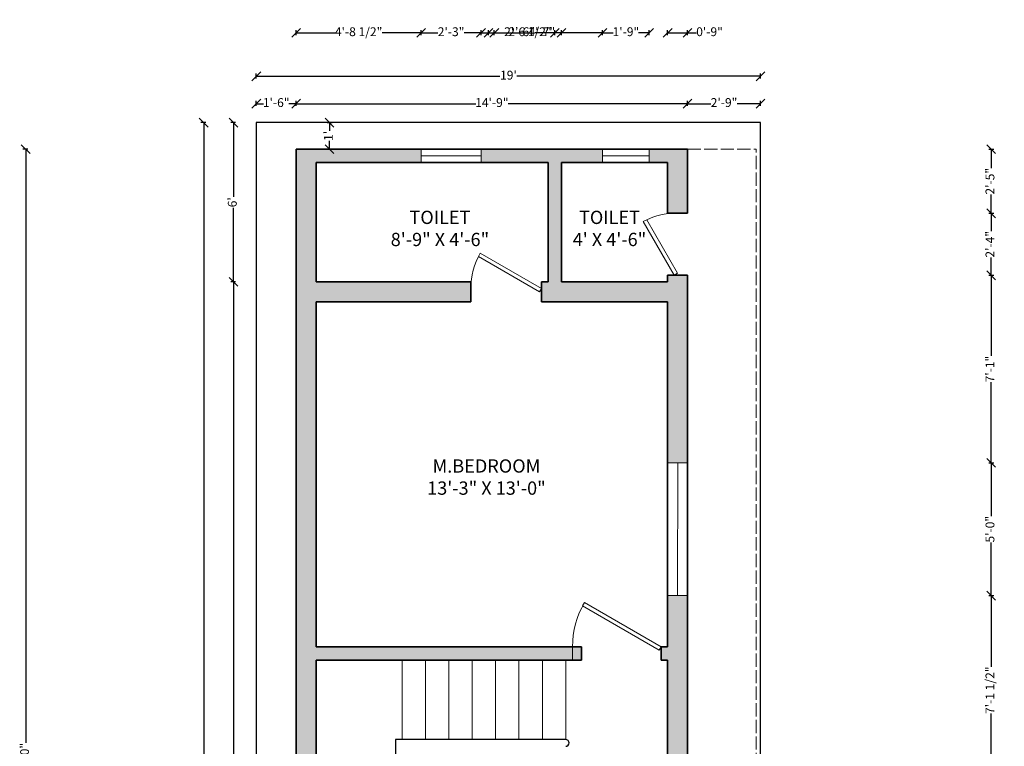
# Model space of a CAD drawing. Units: inches. Extents: x 2349 to 2798, y 397 to 1271.
# Tile 3 of 3: x 2353 to 2798, y 943 to 1271. Entities that reach past the tile are written whole.
import ezdxf

# ---------------------------------------------------------------- set-up
doc = ezdxf.new("R2010")
doc.units = ezdxf.units.IN
doc.linetypes.add('ACAD_ISO02W100', pattern=[15, 12, -3])
for name, color, linetype, lineweight in [('A-ANNO-DIMS', 2, 'Continuous', 18), ('A-AREA-IDEN', 7, 'Continuous', 18), ('A-DOOR', 4, 'Continuous', 18), ('A-FLOR-HRAL', 132, 'Continuous', 25), ('A-FLOR-OVHD', 253, 'ACAD_ISO02W100', 13), ('A-FLOR-STRS', 8, 'Continuous', 18), ('A-GLAZ', 4, 'Continuous', 18), ('A-WALL', 7, 'Continuous', 35), ('A-WALL-PATT', 8, 'Continuous', 13), ('C-PROP', 7, 'Continuous', 25)]:
    doc.layers.add(name, color=color, linetype=linetype, lineweight=lineweight)
doc.styles.get("Standard").update_dxf_attribs({"font": 'arial.ttf'})
doc.dimstyles.new('ISO-25', dxfattribs={"dimtxt": 4, "dimasz": 4, "dimexe": 1.25, "dimexo": 1, "dimtad": 0, "dimdec": 1, "dimlunit": 3, "dimtxsty": 'Standard', "dimblk": 'OBLIQUE', "dimcen": 2.5, "dimclrd": 1, "dimclrt": 3, "dimadec": 0, "dimazin": 0, "dimtfac": 1, "dimtdec": 1, "dimtmove": 0, "dimatfit": 3, "dimfxl": 1, "dimfxlon": 1, "dimarcsym": 0})

# ---------------------------------------------------------------- blocks, each defined once
blk = doc.blocks.new('_Oblique')
at = {"color": 0, "linetype": 'ByBlock', "lineweight": -2}
blk.add_line((-0.5, -0.5), (0.5, 0.5), dxfattribs=at)
blk = doc.blocks.new('*D2')
at = {"layer": 'A-ANNO-DIMS', "color": 0, "lineweight": -2, "transparency": 16777216}
for p, q in [((2491.82, 1224.52), (2494.07, 1224.52)), ((2492.82, 1224.52), (2492.82, 1220.79)), ((2492.82, 1212.52), (2492.82, 1216.24)), ((2491.82, 1212.52), (2494.07, 1212.52))]:
    blk.add_line(p, q, dxfattribs=at)
at = {"layer": 'Defpoints', "color": 0, "transparency": 16777216}
for p in [(2477.73, 1224.52), (2492.82, 1224.52), (2477.73, 1212.52)]:
    blk.add_point(p, dxfattribs=at)
at = {"layer": 'A-ANNO-DIMS', "color": 0, "lineweight": -2, "transparency": 16777216, "xscale": 4, "yscale": 4, "zscale": 4}
for p, rotation in [((2492.82, 1224.52), 90), ((2492.82, 1212.52), 270)]:
    blk.add_blockref('_Oblique', p, dxfattribs=dict(at, rotation=rotation))
at = {"layer": 'A-ANNO-DIMS', "color": 0, "transparency": 16777216, "insert": (2492.82, 1218.52), "char_height": 4, "attachment_point": 5, "rotation": 90}
blk.add_mtext("1'", dxfattribs=at)
blk = doc.blocks.new('*D3')
at = {"layer": 'A-ANNO-DIMS', "color": 0, "lineweight": -2, "transparency": 16777216}
for p, q in [((2459.73, 1232.09), (2459.73, 1234.34)), ((2477.73, 1232.09), (2477.73, 1234.34)), ((2459.73, 1233.09), (2462.98, 1233.09)), ((2477.73, 1233.09), (2474.48, 1233.09))]:
    blk.add_line(p, q, dxfattribs=at)
at = {"layer": 'Defpoints', "color": 0, "transparency": 16777216}
for p in [(2477.73, 1233.09), (2459.73, 1224.52), (2477.73, 1224.52)]:
    blk.add_point(p, dxfattribs=at)
at = {"layer": 'A-ANNO-DIMS', "color": 0, "lineweight": -2, "transparency": 16777216, "xscale": 4, "yscale": 4, "zscale": 4, "rotation": 180}
blk.add_blockref('_Oblique', (2459.73, 1233.09), dxfattribs=at)
at = {"layer": 'A-ANNO-DIMS', "color": 0, "lineweight": -2, "transparency": 16777216, "xscale": 4, "yscale": 4, "zscale": 4}
blk.add_blockref('_Oblique', (2477.73, 1233.09), dxfattribs=at)
at = {"layer": 'A-ANNO-DIMS', "color": 0, "transparency": 16777216, "insert": (2468.73, 1233.09), "char_height": 4, "attachment_point": 5}
blk.add_mtext('1\'-6"', dxfattribs=at)
blk = doc.blocks.new('*D4')
at = {"layer": 'A-ANNO-DIMS', "color": 0, "lineweight": -2, "transparency": 16777216}
for p, q in [((2477.73, 1232.09), (2477.73, 1234.34)), ((2654.73, 1232.09), (2654.73, 1234.34)), ((2477.73, 1233.09), (2558.92, 1233.09)), ((2654.73, 1233.09), (2573.54, 1233.09))]:
    blk.add_line(p, q, dxfattribs=at)
at = {"layer": 'Defpoints', "color": 0, "transparency": 16777216}
for p in [(2654.73, 1233.09), (2477.73, 1224.52), (2654.73, 1226.53)]:
    blk.add_point(p, dxfattribs=at)
at = {"layer": 'A-ANNO-DIMS', "color": 0, "lineweight": -2, "transparency": 16777216, "xscale": 4, "yscale": 4, "zscale": 4, "rotation": 180}
blk.add_blockref('_Oblique', (2477.73, 1233.09), dxfattribs=at)
at = {"layer": 'A-ANNO-DIMS', "color": 0, "lineweight": -2, "transparency": 16777216, "xscale": 4, "yscale": 4, "zscale": 4}
blk.add_blockref('_Oblique', (2654.73, 1233.09), dxfattribs=at)
at = {"layer": 'A-ANNO-DIMS', "color": 0, "transparency": 16777216, "insert": (2566.23, 1233.09), "char_height": 4, "attachment_point": 5}
blk.add_mtext('14\'-9"', dxfattribs=at)
blk = doc.blocks.new('*D5')
at = {"layer": 'A-ANNO-DIMS', "color": 0, "lineweight": -2, "transparency": 16777216}
for p, q in [((2654.73, 1232.09), (2654.73, 1234.34)), ((2687.73, 1232.09), (2687.73, 1234.34)), ((2654.73, 1233.09), (2665.26, 1233.09)), ((2687.73, 1233.09), (2677.21, 1233.09))]:
    blk.add_line(p, q, dxfattribs=at)
at = {"layer": 'Defpoints', "color": 0, "transparency": 16777216}
for p in [(2687.73, 1233.09), (2654.73, 1226.53), (2687.73, 1224.52)]:
    blk.add_point(p, dxfattribs=at)
at = {"layer": 'A-ANNO-DIMS', "color": 0, "lineweight": -2, "transparency": 16777216, "xscale": 4, "yscale": 4, "zscale": 4, "rotation": 180}
blk.add_blockref('_Oblique', (2654.73, 1233.09), dxfattribs=at)
at = {"layer": 'A-ANNO-DIMS', "color": 0, "lineweight": -2, "transparency": 16777216, "xscale": 4, "yscale": 4, "zscale": 4}
blk.add_blockref('_Oblique', (2687.73, 1233.09), dxfattribs=at)
at = {"layer": 'A-ANNO-DIMS', "color": 0, "transparency": 16777216, "insert": (2671.23, 1233.09), "char_height": 4, "attachment_point": 5}
blk.add_mtext('2\'-9"', dxfattribs=at)
blk = doc.blocks.new('*D6')
at = {"layer": 'A-ANNO-DIMS', "color": 0, "lineweight": -2, "transparency": 16777216}
for p, q in [((2459.73, 1244.48), (2459.73, 1246.73)), ((2687.73, 1244.48), (2687.73, 1246.73)), ((2459.73, 1245.48), (2569.9, 1245.48)), ((2687.73, 1245.48), (2577.56, 1245.48))]:
    blk.add_line(p, q, dxfattribs=at)
at = {"layer": 'Defpoints', "color": 0, "transparency": 16777216}
for p in [(2687.73, 1245.48), (2459.73, 1224.52), (2687.73, 1224.52)]:
    blk.add_point(p, dxfattribs=at)
at = {"layer": 'A-ANNO-DIMS', "color": 0, "lineweight": -2, "transparency": 16777216, "xscale": 4, "yscale": 4, "zscale": 4, "rotation": 180}
blk.add_blockref('_Oblique', (2459.73, 1245.48), dxfattribs=at)
at = {"layer": 'A-ANNO-DIMS', "color": 0, "lineweight": -2, "transparency": 16777216, "xscale": 4, "yscale": 4, "zscale": 4}
blk.add_blockref('_Oblique', (2687.73, 1245.48), dxfattribs=at)
at = {"layer": 'A-ANNO-DIMS', "color": 0, "transparency": 16777216, "insert": (2573.73, 1245.48), "char_height": 4, "attachment_point": 5}
blk.add_mtext("19'", dxfattribs=at)
blk = doc.blocks.new('*D7')
at = {"layer": 'A-ANNO-DIMS', "color": 0, "lineweight": -2, "transparency": 16777216}
for p, q in [((2450.39, 1224.52), (2448.14, 1224.52)), ((2449.39, 1224.52), (2449.39, 1190.99)), ((2449.39, 1152.52), (2449.39, 1186.04)), ((2450.39, 1152.52), (2448.14, 1152.52))]:
    blk.add_line(p, q, dxfattribs=at)
at = {"layer": 'Defpoints', "color": 0, "transparency": 16777216}
for p in [(2459.73, 1224.52), (2449.39, 1152.52), (2459.73, 1152.52)]:
    blk.add_point(p, dxfattribs=at)
at = {"layer": 'A-ANNO-DIMS', "color": 0, "lineweight": -2, "transparency": 16777216, "xscale": 4, "yscale": 4, "zscale": 4}
for p, rotation in [((2449.39, 1224.52), 90), ((2449.39, 1152.52), 270)]:
    blk.add_blockref('_Oblique', p, dxfattribs=dict(at, rotation=rotation))
at = {"layer": 'A-ANNO-DIMS', "color": 0, "transparency": 16777216, "insert": (2449.39, 1188.52), "char_height": 4, "attachment_point": 5, "rotation": 90}
blk.add_mtext("6'", dxfattribs=at)
blk = doc.blocks.new('*D8')
at = {"layer": 'A-ANNO-DIMS', "color": 0, "lineweight": -2, "transparency": 16777216}
for p, q in [((2450.39, 1152.52), (2448.14, 1152.52)), ((2449.39, 1152.52), (2449.39, 914.09)), ((2449.39, 660.52), (2449.39, 898.94)), ((2448.39, 660.52), (2450.64, 660.52))]:
    blk.add_line(p, q, dxfattribs=at)
at = {"layer": 'Defpoints', "color": 0, "transparency": 16777216}
for p in [(2459.73, 1152.52), (2435.42, 660.52), (2449.39, 660.52)]:
    blk.add_point(p, dxfattribs=at)
at = {"layer": 'A-ANNO-DIMS', "color": 0, "lineweight": -2, "transparency": 16777216, "xscale": 4, "yscale": 4, "zscale": 4}
for p, rotation in [((2449.39, 1152.52), 90), ((2449.39, 660.52), 270)]:
    blk.add_blockref('_Oblique', p, dxfattribs=dict(at, rotation=rotation))
at = {"layer": 'A-ANNO-DIMS', "color": 0, "transparency": 16777216, "insert": (2449.39, 906.52), "char_height": 4, "attachment_point": 5, "rotation": 90}
blk.add_mtext('40\'-6"', dxfattribs=at)
blk = doc.blocks.new('*D10')
at = {"layer": 'A-ANNO-DIMS', "color": 0, "lineweight": -2, "transparency": 16777216}
for p, q in [((2436.96, 1224.52), (2434.71, 1224.52)), ((2435.96, 1224.52), (2435.96, 868.55)), ((2435.96, 504.52), (2435.96, 860.49)), ((2436.96, 504.52), (2434.71, 504.52))]:
    blk.add_line(p, q, dxfattribs=at)
at = {"layer": 'Defpoints', "color": 0, "transparency": 16777216}
for p in [(2459.73, 1224.52), (2435.96, 504.52), (2459.73, 504.52)]:
    blk.add_point(p, dxfattribs=at)
at = {"layer": 'A-ANNO-DIMS', "color": 0, "lineweight": -2, "transparency": 16777216, "xscale": 4, "yscale": 4, "zscale": 4}
for p, rotation in [((2435.96, 1224.52), 90), ((2435.96, 504.52), 270)]:
    blk.add_blockref('_Oblique', p, dxfattribs=dict(at, rotation=rotation))
at = {"layer": 'A-ANNO-DIMS', "color": 0, "transparency": 16777216, "insert": (2435.96, 864.52), "char_height": 4, "attachment_point": 5, "rotation": 90}
blk.add_mtext("60'", dxfattribs=at)
blk = doc.blocks.new('*U13')
for p, q in [((0, 0), (0, -6)), ((28, 0), (28, -6))]:
    blk.add_line(p, q)
blk.add_lwpolyline([(0, 0), (24.25, 14), (25.12, 12.48), (0.87, -1.52)], close=True)
blk.add_arc((0, 0), 28, 0, 30)
blk = doc.blocks.new('*U14')
for p, q in [((0, 0), (0, -6)), ((-40, 0), (-40, -6))]:
    blk.add_line(p, q)
blk.add_lwpolyline([(0, 0), (-34.64, 20), (-35.52, 18.48), (-0.88, -1.52)], close=True)
blk.add_arc((0, 0), 40, 150, 180)
blk = doc.blocks.new('*U17')
for p, q in [((0, 0), (0, -6)), ((-32, 0), (-32, -6))]:
    blk.add_line(p, q)
blk.add_lwpolyline([(0, 0), (-27.71, 16), (-28.59, 14.48), (-0.88, -1.52)], close=True)
blk.add_arc((0, 0), 32, 150, 180)
blk = doc.blocks.new('*D19')
at = {"layer": 'A-ANNO-DIMS', "color": 0, "lineweight": -2, "transparency": 16777216}
for p, q in [((2356.46, 1212.52), (2354.21, 1212.52)), ((2356.46, 660.52), (2354.21, 660.52))]:
    blk.add_line(p, q, dxfattribs=at)
at = {"layer": 'A-ANNO-DIMS', "color": 1, "lineweight": -2, "transparency": 16777216}
for p, q in [((2355.46, 1212.52), (2355.46, 944.09)), ((2355.46, 660.52), (2355.46, 928.94))]:
    blk.add_line(p, q, dxfattribs=at)
at = {"layer": 'Defpoints', "color": 0, "transparency": 16777216}
for p in [(2355.46, 1212.52), (2477.73, 1212.52), (2477.73, 660.52)]:
    blk.add_point(p, dxfattribs=at)
at = {"layer": 'A-ANNO-DIMS', "color": 1, "lineweight": -2, "transparency": 16777216, "xscale": 4, "yscale": 4, "zscale": 4}
for p, rotation in [((2355.46, 1212.52), 90), ((2355.46, 660.52), 270)]:
    blk.add_blockref('_Oblique', p, dxfattribs=dict(at, rotation=rotation))
at = {"layer": 'A-ANNO-DIMS', "color": 3, "transparency": 16777216, "insert": (2355.46, 936.52), "char_height": 4, "attachment_point": 5, "rotation": 90}
blk.add_mtext('46\'-0"', dxfattribs=at)
blk = doc.blocks.new('*D23')
at = {"layer": 'A-ANNO-DIMS', "color": 0, "lineweight": -2, "transparency": 16777216}
for p, q in [((2790.99, 1010.67), (2793.24, 1010.67)), ((2790.99, 925.07), (2793.24, 925.07))]:
    blk.add_line(p, q, dxfattribs=at)
at = {"layer": 'A-ANNO-DIMS', "color": 1, "lineweight": -2, "transparency": 16777216}
for p, q in [((2791.99, 1010.67), (2791.99, 978.45)), ((2791.99, 925.07), (2791.99, 957.28))]:
    blk.add_line(p, q, dxfattribs=at)
at = {"layer": 'Defpoints', "color": 0, "transparency": 16777216}
for p in [(2654.73, 1010.67), (2791.99, 1010.67), (2654.73, 925.07)]:
    blk.add_point(p, dxfattribs=at)
at = {"layer": 'A-ANNO-DIMS', "color": 1, "lineweight": -2, "transparency": 16777216, "xscale": 4, "yscale": 4, "zscale": 4}
for p, rotation in [((2791.99, 1010.67), 90), ((2791.99, 925.07), 270)]:
    blk.add_blockref('_Oblique', p, dxfattribs=dict(at, rotation=rotation))
at = {"layer": 'A-ANNO-DIMS', "color": 3, "transparency": 16777216, "insert": (2791.99, 967.87), "char_height": 4, "attachment_point": 5, "rotation": 90}
blk.add_mtext('7\'-1 1/2"', dxfattribs=at)
blk = doc.blocks.new('*D24')
at = {"layer": 'A-ANNO-DIMS', "color": 0, "lineweight": -2, "transparency": 16777216}
for p, q in [((2790.99, 1070.67), (2793.24, 1070.67)), ((2790.99, 1010.67), (2793.24, 1010.67))]:
    blk.add_line(p, q, dxfattribs=at)
at = {"layer": 'A-ANNO-DIMS', "color": 1, "lineweight": -2, "transparency": 16777216}
for p, q in [((2791.99, 1070.67), (2791.99, 1046.61)), ((2791.99, 1010.67), (2791.99, 1034.72))]:
    blk.add_line(p, q, dxfattribs=at)
at = {"layer": 'Defpoints', "color": 0, "transparency": 16777216}
for p in [(2654.73, 1070.67), (2791.99, 1070.67), (2654.73, 1010.67)]:
    blk.add_point(p, dxfattribs=at)
at = {"layer": 'A-ANNO-DIMS', "color": 1, "lineweight": -2, "transparency": 16777216, "xscale": 4, "yscale": 4, "zscale": 4}
for p, rotation in [((2791.99, 1070.67), 90), ((2791.99, 1010.67), 270)]:
    blk.add_blockref('_Oblique', p, dxfattribs=dict(at, rotation=rotation))
at = {"layer": 'A-ANNO-DIMS', "color": 3, "transparency": 16777216, "insert": (2791.99, 1040.67), "char_height": 4, "attachment_point": 5, "rotation": 90}
blk.add_mtext('5\'-0"', dxfattribs=at)
blk = doc.blocks.new('*D25')
at = {"layer": 'A-ANNO-DIMS', "color": 0, "lineweight": -2, "transparency": 16777216}
for p, q in [((2790.99, 1155.52), (2793.24, 1155.52)), ((2790.99, 1070.67), (2793.24, 1070.67))]:
    blk.add_line(p, q, dxfattribs=at)
at = {"layer": 'A-ANNO-DIMS', "color": 1, "lineweight": -2, "transparency": 16777216}
for p, q in [((2791.99, 1155.52), (2791.99, 1119.02)), ((2791.99, 1070.67), (2791.99, 1107.17))]:
    blk.add_line(p, q, dxfattribs=at)
at = {"layer": 'Defpoints', "color": 0, "transparency": 16777216}
for p in [(2654.73, 1155.52), (2791.99, 1155.52), (2654.73, 1070.67)]:
    blk.add_point(p, dxfattribs=at)
at = {"layer": 'A-ANNO-DIMS', "color": 1, "lineweight": -2, "transparency": 16777216, "xscale": 4, "yscale": 4, "zscale": 4}
for p, rotation in [((2791.99, 1155.52), 90), ((2791.99, 1070.67), 270)]:
    blk.add_blockref('_Oblique', p, dxfattribs=dict(at, rotation=rotation))
at = {"layer": 'A-ANNO-DIMS', "color": 3, "transparency": 16777216, "insert": (2791.99, 1113.09), "char_height": 4, "attachment_point": 5, "rotation": 90}
blk.add_mtext('7\'-1"', dxfattribs=at)
blk = doc.blocks.new('*D26')
at = {"layer": 'A-ANNO-DIMS', "color": 0, "lineweight": -2, "transparency": 16777216}
for p, q in [((2790.99, 1183.52), (2793.24, 1183.52)), ((2790.99, 1155.52), (2793.24, 1155.52))]:
    blk.add_line(p, q, dxfattribs=at)
at = {"layer": 'A-ANNO-DIMS', "color": 1, "lineweight": -2, "transparency": 16777216}
for p, q in [((2791.99, 1183.52), (2791.99, 1175.49)), ((2791.99, 1155.52), (2791.99, 1163.54))]:
    blk.add_line(p, q, dxfattribs=at)
at = {"layer": 'Defpoints', "color": 0, "transparency": 16777216}
for p in [(2654.73, 1183.52), (2791.99, 1183.52), (2654.73, 1155.52)]:
    blk.add_point(p, dxfattribs=at)
at = {"layer": 'A-ANNO-DIMS', "color": 1, "lineweight": -2, "transparency": 16777216, "xscale": 4, "yscale": 4, "zscale": 4}
for p, rotation in [((2791.99, 1183.52), 90), ((2791.99, 1155.52), 270)]:
    blk.add_blockref('_Oblique', p, dxfattribs=dict(at, rotation=rotation))
at = {"layer": 'A-ANNO-DIMS', "color": 3, "transparency": 16777216, "insert": (2791.99, 1169.52), "char_height": 4, "attachment_point": 5, "rotation": 90}
blk.add_mtext('2\'-4"', dxfattribs=at)
blk = doc.blocks.new('*D27')
at = {"layer": 'A-ANNO-DIMS', "color": 0, "lineweight": -2, "transparency": 16777216}
for p, q in [((2790.99, 1212.52), (2793.24, 1212.52)), ((2790.99, 1183.52), (2793.24, 1183.52))]:
    blk.add_line(p, q, dxfattribs=at)
at = {"layer": 'A-ANNO-DIMS', "color": 1, "lineweight": -2, "transparency": 16777216}
for p, q in [((2791.99, 1212.52), (2791.99, 1203.99)), ((2791.99, 1183.52), (2791.99, 1192.04))]:
    blk.add_line(p, q, dxfattribs=at)
at = {"layer": 'Defpoints', "color": 0, "transparency": 16777216}
for p in [(2654.73, 1212.52), (2791.99, 1212.52), (2654.73, 1183.52)]:
    blk.add_point(p, dxfattribs=at)
at = {"layer": 'A-ANNO-DIMS', "color": 1, "lineweight": -2, "transparency": 16777216, "xscale": 4, "yscale": 4, "zscale": 4}
for p, rotation in [((2791.99, 1212.52), 90), ((2791.99, 1183.52), 270)]:
    blk.add_blockref('_Oblique', p, dxfattribs=dict(at, rotation=rotation))
at = {"layer": 'A-ANNO-DIMS', "color": 3, "transparency": 16777216, "insert": (2791.99, 1198.02), "char_height": 4, "attachment_point": 5, "rotation": 90}
blk.add_mtext('2\'-5"', dxfattribs=at)
blk = doc.blocks.new('*D32')
at = {"layer": 'A-ANNO-DIMS', "color": 0, "lineweight": -2, "transparency": 16777216}
for p, q in [((2606.73, 403.67), (2606.73, 401.42)), ((2642.73, 403.67), (2642.73, 401.42))]:
    blk.add_line(p, q, dxfattribs=at)
at = {"layer": 'A-ANNO-DIMS', "color": 1, "lineweight": -2, "transparency": 16777216}
for p, q in [((2606.73, 402.67), (2618.79, 402.67)), ((2642.73, 402.67), (2630.67, 402.67))]:
    blk.add_line(p, q, dxfattribs=at)
at = {"layer": 'Defpoints', "color": 0, "transparency": 16777216}
for p in [(2606.73, 981.52), (2642.73, 981.52), (2642.73, 402.67)]:
    blk.add_point(p, dxfattribs=at)
at = {"layer": 'A-ANNO-DIMS', "color": 1, "lineweight": -2, "transparency": 16777216, "xscale": 4, "yscale": 4, "zscale": 4, "rotation": 180}
blk.add_blockref('_Oblique', (2606.73, 402.67), dxfattribs=at)
at = {"layer": 'A-ANNO-DIMS', "color": 1, "lineweight": -2, "transparency": 16777216, "xscale": 4, "yscale": 4, "zscale": 4}
blk.add_blockref('_Oblique', (2642.73, 402.67), dxfattribs=at)
at = {"layer": 'A-ANNO-DIMS', "color": 3, "transparency": 16777216, "insert": (2624.73, 402.67), "char_height": 4, "attachment_point": 5}
blk.add_mtext('3\'-0"', dxfattribs=at)
blk = doc.blocks.new('*D33')
at = {"layer": 'A-ANNO-DIMS', "color": 0, "lineweight": -2, "transparency": 16777216}
for p, q in [((2556.73, 403.67), (2556.73, 401.42)), ((2588.73, 403.67), (2588.73, 401.42))]:
    blk.add_line(p, q, dxfattribs=at)
at = {"layer": 'A-ANNO-DIMS', "color": 1, "lineweight": -2, "transparency": 16777216}
for p, q in [((2556.73, 402.67), (2566.76, 402.67)), ((2588.73, 402.67), (2578.71, 402.67))]:
    blk.add_line(p, q, dxfattribs=at)
at = {"layer": 'Defpoints', "color": 0, "transparency": 16777216}
for p in [(2556.73, 1143.52), (2588.73, 1143.52), (2588.73, 402.67)]:
    blk.add_point(p, dxfattribs=at)
at = {"layer": 'A-ANNO-DIMS', "color": 1, "lineweight": -2, "transparency": 16777216, "xscale": 4, "yscale": 4, "zscale": 4, "rotation": 180}
blk.add_blockref('_Oblique', (2556.73, 402.67), dxfattribs=at)
at = {"layer": 'A-ANNO-DIMS', "color": 1, "lineweight": -2, "transparency": 16777216, "xscale": 4, "yscale": 4, "zscale": 4}
blk.add_blockref('_Oblique', (2588.73, 402.67), dxfattribs=at)
at = {"layer": 'A-ANNO-DIMS', "color": 3, "transparency": 16777216, "insert": (2572.73, 402.67), "char_height": 4, "attachment_point": 5}
blk.add_mtext('2\'-8"', dxfattribs=at)
blk = doc.blocks.new('*D34')
at = {"layer": 'A-ANNO-DIMS', "color": 0, "lineweight": -2, "transparency": 16777216}
for p, q in [((2477.73, 1264.12), (2477.73, 1266.37)), ((2534.27, 1264.12), (2534.27, 1266.37))]:
    blk.add_line(p, q, dxfattribs=at)
at = {"layer": 'A-ANNO-DIMS', "color": 1, "lineweight": -2, "transparency": 16777216}
for p, q in [((2477.73, 1265.12), (2495.32, 1265.12)), ((2534.27, 1265.12), (2516.68, 1265.12))]:
    blk.add_line(p, q, dxfattribs=at)
at = {"layer": 'Defpoints', "color": 0, "transparency": 16777216}
for p in [(2534.27, 1265.12), (2477.73, 1212.52), (2534.27, 1212.52)]:
    blk.add_point(p, dxfattribs=at)
at = {"layer": 'A-ANNO-DIMS', "color": 1, "lineweight": -2, "transparency": 16777216, "xscale": 4, "yscale": 4, "zscale": 4, "rotation": 180}
blk.add_blockref('_Oblique', (2477.73, 1265.12), dxfattribs=at)
at = {"layer": 'A-ANNO-DIMS', "color": 1, "lineweight": -2, "transparency": 16777216, "xscale": 4, "yscale": 4, "zscale": 4}
blk.add_blockref('_Oblique', (2534.27, 1265.12), dxfattribs=at)
at = {"layer": 'A-ANNO-DIMS', "color": 3, "transparency": 16777216, "insert": (2506, 1265.12), "char_height": 4, "attachment_point": 5}
blk.add_mtext('4\'-8 1/2"', dxfattribs=at)
blk = doc.blocks.new('*D35')
at = {"layer": 'A-ANNO-DIMS', "color": 0, "lineweight": -2, "transparency": 16777216}
for p, q in [((2534.27, 1264.12), (2534.27, 1266.37)), ((2561.36, 1264.12), (2561.36, 1266.37))]:
    blk.add_line(p, q, dxfattribs=at)
at = {"layer": 'A-ANNO-DIMS', "color": 1, "lineweight": -2, "transparency": 16777216}
for p, q in [((2534.27, 1265.12), (2541.84, 1265.12)), ((2561.36, 1265.12), (2553.79, 1265.12))]:
    blk.add_line(p, q, dxfattribs=at)
at = {"layer": 'Defpoints', "color": 0, "transparency": 16777216}
for p in [(2561.36, 1265.12), (2534.27, 1212.52), (2561.36, 1212.52)]:
    blk.add_point(p, dxfattribs=at)
at = {"layer": 'A-ANNO-DIMS', "color": 1, "lineweight": -2, "transparency": 16777216, "xscale": 4, "yscale": 4, "zscale": 4, "rotation": 180}
blk.add_blockref('_Oblique', (2534.27, 1265.12), dxfattribs=at)
at = {"layer": 'A-ANNO-DIMS', "color": 1, "lineweight": -2, "transparency": 16777216, "xscale": 4, "yscale": 4, "zscale": 4}
blk.add_blockref('_Oblique', (2561.36, 1265.12), dxfattribs=at)
at = {"layer": 'A-ANNO-DIMS', "color": 3, "transparency": 16777216, "insert": (2547.81, 1265.12), "char_height": 4, "attachment_point": 5}
blk.add_mtext('2\'-3"', dxfattribs=at)
blk = doc.blocks.new('*D36')
at = {"layer": 'A-ANNO-DIMS', "color": 0, "lineweight": -2, "transparency": 16777216}
for p, q in [((2561.36, 1264.12), (2561.36, 1266.37)), ((2616.29, 1264.12), (2616.29, 1266.37))]:
    blk.add_line(p, q, dxfattribs=at)
at = {"layer": 'A-ANNO-DIMS', "color": 1, "lineweight": -2, "transparency": 16777216}
for p, q in [((2561.36, 1265.12), (2582.8, 1265.12)), ((2616.29, 1265.12), (2594.84, 1265.12))]:
    blk.add_line(p, q, dxfattribs=at)
at = {"layer": 'Defpoints', "color": 0, "transparency": 16777216}
for p in [(2616.29, 1265.12), (2561.36, 1212.52), (2616.29, 1212.52)]:
    blk.add_point(p, dxfattribs=at)
at = {"layer": 'A-ANNO-DIMS', "color": 1, "lineweight": -2, "transparency": 16777216, "xscale": 4, "yscale": 4, "zscale": 4, "rotation": 180}
blk.add_blockref('_Oblique', (2561.36, 1265.12), dxfattribs=at)
at = {"layer": 'A-ANNO-DIMS', "color": 1, "lineweight": -2, "transparency": 16777216, "xscale": 4, "yscale": 4, "zscale": 4}
blk.add_blockref('_Oblique', (2616.29, 1265.12), dxfattribs=at)
at = {"layer": 'A-ANNO-DIMS', "color": 3, "transparency": 16777216, "insert": (2588.82, 1265.12), "char_height": 4, "attachment_point": 5}
blk.add_mtext('4\'-7"', dxfattribs=at)
blk = doc.blocks.new('*D37')
at = {"layer": 'A-ANNO-DIMS', "color": 0, "lineweight": -2, "transparency": 16777216}
for p, q in [((2616.29, 1264.12), (2616.29, 1266.37)), ((2637.4, 1264.12), (2637.4, 1266.37))]:
    blk.add_line(p, q, dxfattribs=at)
at = {"layer": 'A-ANNO-DIMS', "color": 1, "lineweight": -2, "transparency": 16777216}
for p, q in [((2616.29, 1265.12), (2621.09, 1265.12)), ((2637.4, 1265.12), (2632.6, 1265.12))]:
    blk.add_line(p, q, dxfattribs=at)
at = {"layer": 'Defpoints', "color": 0, "transparency": 16777216}
for p in [(2637.4, 1265.12), (2616.29, 1212.52), (2637.4, 1212.52)]:
    blk.add_point(p, dxfattribs=at)
at = {"layer": 'A-ANNO-DIMS', "color": 1, "lineweight": -2, "transparency": 16777216, "xscale": 4, "yscale": 4, "zscale": 4, "rotation": 180}
blk.add_blockref('_Oblique', (2616.29, 1265.12), dxfattribs=at)
at = {"layer": 'A-ANNO-DIMS', "color": 1, "lineweight": -2, "transparency": 16777216, "xscale": 4, "yscale": 4, "zscale": 4}
blk.add_blockref('_Oblique', (2637.4, 1265.12), dxfattribs=at)
at = {"layer": 'A-ANNO-DIMS', "color": 3, "transparency": 16777216, "insert": (2626.85, 1265.12), "char_height": 4, "attachment_point": 5}
blk.add_mtext('1\'-9"', dxfattribs=at)
blk = doc.blocks.new('*D41')
at = {"layer": 'A-ANNO-DIMS', "color": 0, "lineweight": -2, "transparency": 16777216}
for p, q in [((2564.73, 1264.12), (2564.73, 1266.37)), ((2594.73, 1264.12), (2594.73, 1266.37))]:
    blk.add_line(p, q, dxfattribs=at)
at = {"layer": 'A-ANNO-DIMS', "color": 1, "lineweight": -2, "transparency": 16777216}
for p, q in [((2564.73, 1265.12), (2573.76, 1265.12)), ((2594.73, 1265.12), (2585.71, 1265.12))]:
    blk.add_line(p, q, dxfattribs=at)
at = {"layer": 'Defpoints', "color": 0, "transparency": 16777216}
for p in [(2594.73, 1265.12), (2564.73, 801.52), (2594.73, 801.52)]:
    blk.add_point(p, dxfattribs=at)
at = {"layer": 'A-ANNO-DIMS', "color": 1, "lineweight": -2, "transparency": 16777216, "xscale": 4, "yscale": 4, "zscale": 4, "rotation": 180}
blk.add_blockref('_Oblique', (2564.73, 1265.12), dxfattribs=at)
at = {"layer": 'A-ANNO-DIMS', "color": 1, "lineweight": -2, "transparency": 16777216, "xscale": 4, "yscale": 4, "zscale": 4}
blk.add_blockref('_Oblique', (2594.73, 1265.12), dxfattribs=at)
at = {"layer": 'A-ANNO-DIMS', "color": 3, "transparency": 16777216, "insert": (2579.73, 1265.12), "char_height": 4, "attachment_point": 5}
blk.add_mtext('2\'-6"', dxfattribs=at)
blk = doc.blocks.new('*D42')
at = {"layer": 'A-ANNO-DIMS', "color": 0, "lineweight": -2, "transparency": 16777216}
for p, q in [((2567.33, 1264.12), (2567.33, 1266.37)), ((2597.73, 1264.12), (2597.73, 1266.37))]:
    blk.add_line(p, q, dxfattribs=at)
at = {"layer": 'A-ANNO-DIMS', "color": 1, "lineweight": -2, "transparency": 16777216}
for p, q in [((2567.33, 1265.12), (2571.89, 1265.12)), ((2597.73, 1265.12), (2593.16, 1265.12))]:
    blk.add_line(p, q, dxfattribs=at)
at = {"layer": 'Defpoints', "color": 0, "transparency": 16777216}
for p in [(2567.33, 1265.12), (2567.33, 697.63), (2597.73, 669.52)]:
    blk.add_point(p, dxfattribs=at)
at = {"layer": 'A-ANNO-DIMS', "color": 1, "lineweight": -2, "transparency": 16777216, "xscale": 4, "yscale": 4, "zscale": 4, "rotation": 180}
blk.add_blockref('_Oblique', (2567.33, 1265.12), dxfattribs=at)
at = {"layer": 'A-ANNO-DIMS', "color": 1, "lineweight": -2, "transparency": 16777216, "xscale": 4, "yscale": 4, "zscale": 4}
blk.add_blockref('_Oblique', (2597.73, 1265.12), dxfattribs=at)
at = {"layer": 'A-ANNO-DIMS', "color": 3, "transparency": 16777216, "insert": (2582.53, 1265.12), "char_height": 4, "attachment_point": 5}
blk.add_mtext('2\'-6 1/2"', dxfattribs=at)
blk = doc.blocks.new('*D44')
at = {"layer": 'A-ANNO-DIMS', "color": 0, "lineweight": -2, "transparency": 16777216}
for p, q in [((2645.73, 1264.12), (2645.73, 1266.37)), ((2654.73, 1264.12), (2654.73, 1266.37))]:
    blk.add_line(p, q, dxfattribs=at)
at = {"layer": 'A-ANNO-DIMS', "color": 1, "lineweight": -2, "transparency": 16777216}
for p, q in [((2645.73, 1265.12), (2654.73, 1265.12)), ((2654.73, 1265.12), (2658.73, 1265.12))]:
    blk.add_line(p, q, dxfattribs=at)
at = {"layer": 'Defpoints', "color": 0, "transparency": 16777216}
for p in [(2654.73, 1265.12), (2645.73, 675.52), (2654.73, 675.52)]:
    blk.add_point(p, dxfattribs=at)
at = {"layer": 'A-ANNO-DIMS', "color": 1, "lineweight": -2, "transparency": 16777216, "xscale": 4, "yscale": 4, "zscale": 4, "rotation": 180}
blk.add_blockref('_Oblique', (2645.73, 1265.12), dxfattribs=at)
at = {"layer": 'A-ANNO-DIMS', "color": 1, "lineweight": -2, "transparency": 16777216, "xscale": 4, "yscale": 4, "zscale": 4}
blk.add_blockref('_Oblique', (2654.73, 1265.12), dxfattribs=at)
at = {"layer": 'A-ANNO-DIMS', "color": 3, "transparency": 16777216, "insert": (2664.67, 1265.12), "char_height": 4, "attachment_point": 5}
blk.add_mtext('0\'-9"', dxfattribs=at)
blk = doc.blocks.new('*D46')
at = {"layer": 'A-ANNO-DIMS', "color": 0, "lineweight": -2, "transparency": 16777216}
for p, q in [((2591.73, 403.67), (2591.73, 401.42)), ((2597.73, 403.67), (2597.73, 401.42))]:
    blk.add_line(p, q, dxfattribs=at)
at = {"layer": 'A-ANNO-DIMS', "color": 1, "lineweight": -2, "transparency": 16777216}
for p, q in [((2591.73, 402.67), (2597.73, 402.67)), ((2597.73, 402.67), (2601.73, 402.67))]:
    blk.add_line(p, q, dxfattribs=at)
at = {"layer": 'Defpoints', "color": 0, "transparency": 16777216}
for p in [(2591.73, 1206.52), (2597.73, 1206.52), (2597.73, 402.67)]:
    blk.add_point(p, dxfattribs=at)
at = {"layer": 'A-ANNO-DIMS', "color": 1, "lineweight": -2, "transparency": 16777216, "xscale": 4, "yscale": 4, "zscale": 4, "rotation": 180}
blk.add_blockref('_Oblique', (2591.73, 402.67), dxfattribs=at)
at = {"layer": 'A-ANNO-DIMS', "color": 1, "lineweight": -2, "transparency": 16777216, "xscale": 4, "yscale": 4, "zscale": 4}
blk.add_blockref('_Oblique', (2597.73, 402.67), dxfattribs=at)
at = {"layer": 'A-ANNO-DIMS', "color": 3, "transparency": 16777216, "insert": (2607.67, 402.67), "char_height": 4, "attachment_point": 5}
blk.add_mtext('0\'-6"', dxfattribs=at)
blk = doc.blocks.new('*D47')
at = {"layer": 'A-ANNO-DIMS', "color": 0, "lineweight": -2, "transparency": 16777216}
for p, q in [((2477.73, 403.67), (2477.73, 401.42)), ((2486.73, 403.67), (2486.73, 401.42))]:
    blk.add_line(p, q, dxfattribs=at)
at = {"layer": 'A-ANNO-DIMS', "color": 1, "lineweight": -2, "transparency": 16777216}
for p, q in [((2477.73, 402.67), (2486.73, 402.67)), ((2486.73, 402.67), (2490.73, 402.67))]:
    blk.add_line(p, q, dxfattribs=at)
at = {"layer": 'Defpoints', "color": 0, "transparency": 16777216}
for p in [(2477.73, 1212.52), (2486.73, 1206.52), (2486.73, 402.67)]:
    blk.add_point(p, dxfattribs=at)
at = {"layer": 'A-ANNO-DIMS', "color": 1, "lineweight": -2, "transparency": 16777216, "xscale": 4, "yscale": 4, "zscale": 4, "rotation": 180}
blk.add_blockref('_Oblique', (2477.73, 402.67), dxfattribs=at)
at = {"layer": 'A-ANNO-DIMS', "color": 1, "lineweight": -2, "transparency": 16777216, "xscale": 4, "yscale": 4, "zscale": 4}
blk.add_blockref('_Oblique', (2486.73, 402.67), dxfattribs=at)
at = {"layer": 'A-ANNO-DIMS', "color": 3, "transparency": 16777216, "insert": (2496.67, 402.67), "char_height": 4, "attachment_point": 5}
blk.add_mtext('0\'-9"', dxfattribs=at)
blk = doc.blocks.new('*D48')
at = {"layer": 'A-ANNO-DIMS', "color": 0, "lineweight": -2, "transparency": 16777216}
for p, q in [((2525.73, 403.67), (2525.73, 401.42)), ((2599.63, 403.67), (2599.63, 401.42))]:
    blk.add_line(p, q, dxfattribs=at)
at = {"layer": 'A-ANNO-DIMS', "color": 1, "lineweight": -2, "transparency": 16777216}
for p, q in [((2525.73, 402.67), (2556.73, 402.67)), ((2599.63, 402.67), (2568.63, 402.67))]:
    blk.add_line(p, q, dxfattribs=at)
at = {"layer": 'Defpoints', "color": 0, "transparency": 16777216}
for p in [(2525.73, 942.52), (2599.63, 942.52), (2599.63, 402.67)]:
    blk.add_point(p, dxfattribs=at)
at = {"layer": 'A-ANNO-DIMS', "color": 1, "lineweight": -2, "transparency": 16777216, "xscale": 4, "yscale": 4, "zscale": 4, "rotation": 180}
blk.add_blockref('_Oblique', (2525.73, 402.67), dxfattribs=at)
at = {"layer": 'A-ANNO-DIMS', "color": 1, "lineweight": -2, "transparency": 16777216, "xscale": 4, "yscale": 4, "zscale": 4}
blk.add_blockref('_Oblique', (2599.63, 402.67), dxfattribs=at)
at = {"layer": 'A-ANNO-DIMS', "color": 3, "transparency": 16777216, "insert": (2562.68, 402.67), "char_height": 4, "attachment_point": 5}
blk.add_mtext('6\'-2"', dxfattribs=at)

msp = doc.modelspace()

# ---------------------------------------------------------------- hatches: boundary and pattern name
at = {"layer": 'A-WALL-PATT'}
h = msp.add_hatch(color=256, dxfattribs=at)
h.dxf.hatch_style = 1
h.paths.add_polyline_path([(2616.29, 1212.52), (2561.36, 1212.52), (2561.36, 1206.52), (2591.73, 1206.52), (2591.73, 1152.52), (2588.73, 1152.52), (2588.73, 1143.52), (2645.73, 1143.52), (2645.73, 1070.67), (2654.73, 1070.67), (2654.73, 1155.52), (2645.73, 1155.52), (2645.73, 1152.52), (2597.73, 1152.52), (2597.73, 1206.52), (2616.29, 1206.52)])
h.paths.add_polyline_path([(2654.73, 1212.52), (2637.4, 1212.52), (2637.4, 1206.52), (2645.73, 1206.52), (2645.73, 1183.52), (2654.73, 1183.52)], flags=17)
h.paths.add_polyline_path([(2520.04, 669.52), (2486.73, 669.52), (2486.73, 795.52), (2525.73, 795.52), (2525.73, 801.52), (2486.73, 801.52), (2477.73, 801.52), (2477.73, 660.52), (2520.04, 660.52)])
h.paths.add_polyline_path([(2486.73, 981.52), (2606.73, 981.52), (2606.73, 987.52), (2486.73, 987.52), (2486.73, 1143.52), (2556.73, 1143.52), (2556.73, 1152.52), (2486.73, 1152.52), (2486.73, 1206.52), (2534.27, 1206.52), (2534.27, 1212.52), (2477.73, 1212.52), (2477.73, 836.92), (2486.73, 836.92)])
h.paths.add_polyline_path([(2597.73, 747.52), (2561.73, 747.52), (2561.73, 795.52), (2564.73, 795.52), (2564.73, 801.52), (2555.73, 801.52), (2555.73, 741.52), (2597.73, 741.52)])
h.paths.add_polyline_path([(2654.73, 1010.67), (2645.73, 1010.67), (2645.73, 987.52), (2642.73, 987.52), (2642.73, 981.52), (2645.73, 981.52), (2645.73, 925.07), (2654.73, 925.07)])
h.paths.add_polyline_path([(2645.73, 858.74), (2645.73, 792.52), (2654.73, 792.52), (2654.73, 858.74)])
h.paths.add_polyline_path([(2603.73, 660.52), (2603.73, 801.52), (2594.73, 801.52), (2594.73, 795.52), (2597.73, 795.52), (2597.73, 669.52), (2559.59, 669.52), (2559.59, 660.52)])

# ---------------------------------------------------------------- linework, layer by layer
at = {"layer": 'A-FLOR-HRAL'}
for p, q in [((2522.73, 945.52), (2522.73, 831.4)), ((2599.63, 945.52), (2522.73, 945.52))]:
    msp.add_line(p, q, dxfattribs=at)
msp.add_arc((2599.63, 944.02), 1.5, 270, 90, dxfattribs=at)
at = {"layer": 'A-FLOR-OVHD', "ltscale": 0.5}
for p in [(2654.73, 1212.52), (2685.73, 588.52)]:
    msp.add_line(p, (2685.73, 1212.52), dxfattribs=at)
at = {"layer": 'A-FLOR-STRS'}
for p, q in [((2525.73, 945.52), (2525.73, 981.52)), ((2536.29, 981.52), (2536.29, 945.52)), ((2546.84, 981.52), (2546.84, 945.52)), ((2557.4, 981.52), (2557.4, 945.52)), ((2567.96, 981.52), (2567.96, 945.52)), ((2578.51, 981.52), (2578.51, 945.52)), ((2589.07, 981.52), (2589.07, 945.52)), ((2599.63, 981.52), (2599.63, 945.52))]:
    msp.add_line(p, q, dxfattribs=at)
at = {"layer": 'A-GLAZ'}
for p, q in [((2534.27, 1206.52), (2534.27, 1212.52)), ((2561.36, 1206.52), (2561.36, 1212.52)), ((2616.29, 1206.52), (2616.29, 1212.52)), ((2637.4, 1206.52), (2637.4, 1212.52)), ((2534.27, 1209.52), (2561.36, 1209.52)), ((2616.29, 1209.52), (2637.4, 1209.52)), ((2645.86, 1070.67), (2654.73, 1070.67)), ((2650.23, 1010.67), (2650.3, 1070.67)), ((2645.73, 1010.67), (2654.73, 1010.67))]:
    msp.add_line(p, q, dxfattribs=at)
at = {"layer": 'A-WALL'}
for p, q in [((2477.73, 1212.52), (2477.73, 660.52)), ((2654.73, 1212.52), (2477.73, 1212.52)), ((2654.73, 1183.52), (2654.73, 1212.52)), ((2486.73, 1206.52), (2486.73, 1152.52)), ((2591.73, 1206.52), (2486.73, 1206.52)), ((2591.73, 1206.52), (2591.73, 1152.52)), ((2645.73, 1206.52), (2597.73, 1206.52)), ((2597.73, 1152.52), (2597.73, 1206.52)), ((2645.73, 1183.52), (2645.73, 1206.52)), ((2645.73, 1183.52), (2654.73, 1183.52)), ((2645.73, 1152.52), (2645.73, 1155.52)), ((2645.73, 1155.52), (2654.73, 1155.52)), ((2654.73, 660.52), (2654.73, 1155.52)), ((2556.73, 1152.52), (2486.73, 1152.52)), ((2556.73, 1152.52), (2556.73, 1143.52)), ((2591.73, 1152.52), (2588.73, 1152.52)), ((2588.73, 1152.52), (2588.73, 1143.52)), ((2645.73, 1152.52), (2597.73, 1152.52)), ((2486.73, 1143.52), (2486.73, 987.52)), ((2556.73, 1143.52), (2486.73, 1143.52)), ((2645.73, 1143.52), (2588.73, 1143.52)), ((2645.73, 987.52), (2645.73, 1143.52)), ((2606.73, 987.52), (2486.73, 987.52)), ((2606.73, 981.52), (2606.73, 987.52)), ((2645.73, 987.52), (2642.73, 987.52)), ((2642.73, 981.52), (2642.73, 987.52)), ((2486.73, 981.52), (2486.73, 801.52)), ((2606.73, 981.52), (2486.73, 981.52)), ((2645.73, 981.52), (2642.73, 981.52)), ((2645.73, 792.52), (2645.73, 981.52))]:
    msp.add_line(p, q, dxfattribs=at)
at = {"layer": 'C-PROP'}
for p, q in [((2687.73, 1224.52), (2459.73, 1224.52)), ((2459.73, 1224.52), (2459.73, 504.52)), ((2687.73, 504.52), (2687.73, 1224.52))]:
    msp.add_line(p, q, dxfattribs=at)

# ---------------------------------------------------------------- block references
at = {"layer": 'A-DOOR', "rotation": 90}
msp.add_blockref('*U13', (2648.73, 1155.52), dxfattribs=at)
at = {"layer": 'A-DOOR'}
for name, p in [('*U17', (2588.73, 1149.52)), ('*U14', (2642.73, 987.52))]:
    msp.add_blockref(name, p, dxfattribs=at)

# ---------------------------------------------------------------- texts
at = {"layer": 'A-AREA-IDEN', "char_height": 6, "attachment_point": 1}
for s, width, insert in [('\\pxqc;TOILET\\P8\'-9" X 4\'-6"', 82.6982, (2501.42, 1184.7)), ('\\pxqc;TOILET\\P4\' X 4\'-6"', 70.6119, (2584.12, 1184.7)), ('\\pxqc;M.BEDROOM\\P13\'-3" X 13\'-0"', 82.6982, (2522.45, 1072.27))]:
    msp.add_mtext_dynamic_manual_height_columns(s, width=width, gutter_width=12.5, heights=[0], dxfattribs=dict(at, insert=insert))

# ---------------------------------------------------------------- dimensions: what is measured, and where the dimension line sits
at = {"layer": 'A-ANNO-DIMS'}
for base, p1, p2, override, picture, middle in [((2534.27, 1265.12), (2477.73, 1212.52), (2534.27, 1212.52), {"dimdec": 1, "dimlfac": 1, "dimrnd": 0, "dimzin": 1, "dimdsep": 46, "dimlunit": 4, "dimfrac": 2}, '*D34', (2506, 1265.12)), ((2567.33, 1265.12), (2597.73, 669.52), (2567.33, 697.63), {"dimdec": 1, "dimlfac": 1, "dimrnd": 0, "dimzin": 1, "dimdsep": 46, "dimlunit": 4, "dimfrac": 2}, '*D42', (2582.53, 1265.12)), ((2561.36, 1265.12), (2534.27, 1212.52), (2561.36, 1212.52), {"dimdec": 1, "dimlfac": 1, "dimrnd": 0, "dimzin": 1, "dimdsep": 46, "dimlunit": 4, "dimfrac": 2}, '*D35', (2547.81, 1265.12)), ((2616.29, 1265.12), (2561.36, 1212.52), (2616.29, 1212.52), {"dimdec": 1, "dimlfac": 1, "dimrnd": 0, "dimzin": 1, "dimdsep": 46, "dimlunit": 4, "dimfrac": 2}, '*D36', (2588.82, 1265.12)), ((2594.73, 1265.12), (2564.73, 801.52), (2594.73, 801.52), {"dimdec": 1, "dimlfac": 1, "dimrnd": 0, "dimzin": 1, "dimdsep": 46, "dimlunit": 4, "dimfrac": 2}, '*D41', (2579.73, 1265.12)), ((2637.4, 1265.12), (2616.29, 1212.52), (2637.4, 1212.52), {"dimdec": 1, "dimlfac": 1, "dimrnd": 0, "dimzin": 1, "dimdsep": 46, "dimlunit": 4, "dimfrac": 2}, '*D37', (2626.85, 1265.12)), ((2654.73, 1265.12), (2645.73, 675.52), (2654.73, 675.52), {"dimdec": 1, "dimlfac": 1, "dimrnd": 0, "dimzin": 1, "dimdsep": 46, "dimlunit": 4, "dimfrac": 2}, '*D44', (2664.67, 1265.12)), ((2687.73, 1245.48), (2459.73, 1224.52), (2687.73, 1224.52), {"dimclrd": 0, "dimclre": 0, "dimclrt": 0}, '*D6', (2573.73, 1245.48)), ((2477.73, 1233.09), (2459.73, 1224.52), (2477.73, 1224.52), {"dimclrd": 0, "dimclre": 0, "dimclrt": 0}, '*D3', (2468.73, 1233.09)), ((2654.73, 1233.09), (2477.73, 1224.52), (2654.73, 1226.53), {"dimclrd": 0, "dimclre": 0, "dimclrt": 0, "dimtmove": 1}, '*D4', (2566.23, 1233.09)), ((2687.73, 1233.09), (2654.73, 1226.53), (2687.73, 1224.52), {"dimclrd": 0, "dimclre": 0, "dimclrt": 0, "dimtmove": 1}, '*D5', (2671.23, 1233.09)), ((2486.73, 402.67), (2477.73, 1212.52), (2486.73, 1206.52), {"dimdec": 1, "dimlfac": 1, "dimrnd": 0, "dimzin": 1, "dimdsep": 46, "dimlunit": 4, "dimfrac": 2}, '*D47', (2496.67, 402.67)), ((2597.73, 402.67), (2591.73, 1206.52), (2597.73, 1206.52), {"dimdec": 1, "dimlfac": 1, "dimrnd": 0, "dimzin": 1, "dimdsep": 46, "dimlunit": 4, "dimfrac": 2}, '*D46', (2607.67, 402.67)), ((2588.73, 402.67), (2556.73, 1143.52), (2588.73, 1143.52), {"dimdec": 1, "dimlfac": 1, "dimrnd": 0, "dimzin": 1, "dimdsep": 46, "dimlunit": 4, "dimfrac": 2}, '*D33', (2572.73, 402.67)), ((2642.73, 402.67), (2606.73, 981.52), (2642.73, 981.52), {"dimdec": 1, "dimlfac": 1, "dimrnd": 0, "dimzin": 1, "dimdsep": 46, "dimlunit": 4, "dimfrac": 2}, '*D32', (2624.73, 402.67)), ((2599.63, 402.67), (2525.73, 942.52), (2599.63, 942.52), {"dimdec": 1, "dimlfac": 1, "dimrnd": 0, "dimzin": 1, "dimdsep": 46, "dimlunit": 4, "dimfrac": 2}, '*D48', (2562.68, 402.67))]:
    dim = msp.add_linear_dim(base=base, p1=p1, p2=p2, dimstyle='ISO-25', override=override, dxfattribs=at)
    dim.commit()
    dim.dimension.update_dxf_attribs({"geometry": picture, "text_midpoint": middle})
for base, p1, p2, override, picture, middle in [((2435.96, 504.52), (2459.73, 1224.52), (2459.73, 504.52), {"dimclrd": 0, "dimclre": 0, "dimclrt": 0}, '*D10', (2435.96, 864.52)), ((2449.39, 1152.52), (2459.73, 1224.52), (2459.73, 1152.52), {"dimclrd": 0, "dimclre": 0, "dimclrt": 0}, '*D7', (2449.39, 1188.52)), ((2492.82, 1224.52), (2477.73, 1212.52), (2477.73, 1224.52), {"dimclrd": 0, "dimclre": 0, "dimclrt": 0}, '*D2', (2492.82, 1218.52)), ((2355.46, 1212.52), (2477.73, 660.52), (2477.73, 1212.52), {"dimdec": 1, "dimlfac": 1, "dimrnd": 0, "dimzin": 1, "dimdsep": 46, "dimlunit": 4, "dimfrac": 2}, '*D19', (2355.46, 936.52)), ((2791.99, 1212.52), (2654.73, 1183.52), (2654.73, 1212.52), {"dimdec": 1, "dimlfac": 1, "dimrnd": 0, "dimzin": 1, "dimdsep": 46, "dimlunit": 4, "dimfrac": 2}, '*D27', (2791.99, 1198.02)), ((2791.99, 1183.52), (2654.73, 1155.52), (2654.73, 1183.52), {"dimdec": 1, "dimlfac": 1, "dimrnd": 0, "dimzin": 1, "dimdsep": 46, "dimlunit": 4, "dimfrac": 2}, '*D26', (2791.99, 1169.52)), ((2791.9928, 1155.5165), (2654.731, 1070.6652), (2654.731, 1155.5165), {"dimdec": 1, "dimlfac": 1, "dimrnd": 0, "dimzin": 1, "dimdsep": 46, "dimlunit": 4, "dimfrac": 2}, '*D25', (2791.9928, 1113.0909)), ((2791.99, 1070.67), (2654.73, 1010.67), (2654.73, 1070.67), {"dimdec": 1, "dimlfac": 1, "dimrnd": 0, "dimzin": 1, "dimdsep": 46, "dimlunit": 4, "dimfrac": 2}, '*D24', (2791.99, 1040.67)), ((2791.99, 1010.67), (2654.73, 925.07), (2654.73, 1010.67), {"dimdec": 1, "dimlfac": 1, "dimrnd": 0, "dimzin": 1, "dimdsep": 46, "dimlunit": 4, "dimfrac": 2}, '*D23', (2791.99, 967.87))]:
    dim = msp.add_linear_dim(base=base, p1=p1, p2=p2, angle=90, dimstyle='ISO-25', override=override, dxfattribs=at)
    dim.commit()
    dim.dimension.update_dxf_attribs({"geometry": picture, "text_midpoint": middle})
dim = msp.add_linear_dim(base=(2449.39, 660.52), p1=(2459.73, 1152.52), p2=(2435.42, 660.52), angle=90, text='40\'-6"', dimstyle='ISO-25', override={"dimclrd": 0, "dimclre": 0, "dimclrt": 0, "dimtmove": 1}, dxfattribs=at)
dim.commit()
dim.dimension.update_dxf_attribs({"geometry": '*D8', "text_midpoint": (2449.39, 906.52)})

doc.saveas('drawing.dxf')
